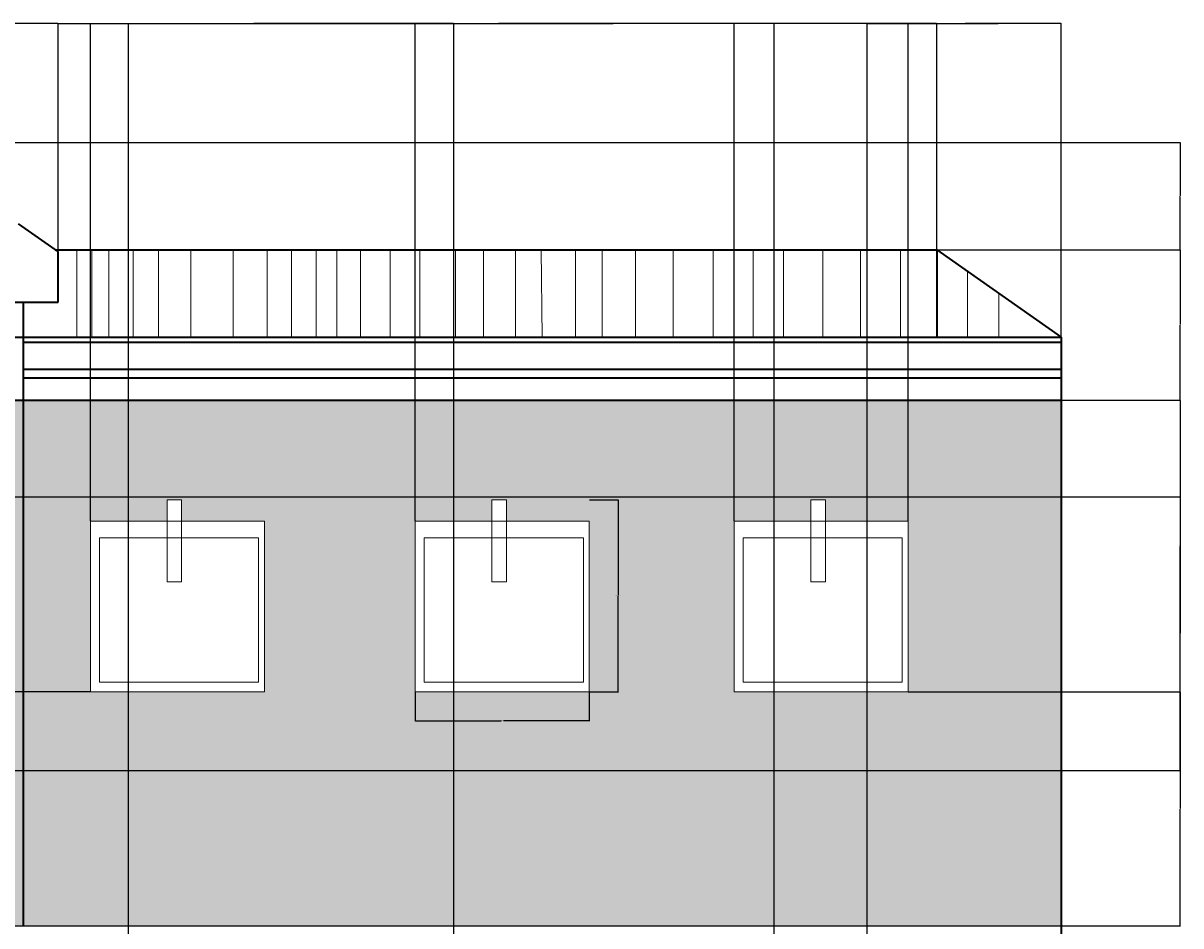
# Model space of a CAD drawing. Units: inches. Extents: x -46 to 1209, y 110 to 778.
# Tile 5 of 5: x 652 to 1209, y 342 to 778. Entities that reach past the tile are written whole.
import ezdxf

# ---------------------------------------------------------------- set-up
doc = ezdxf.new("R2010")
doc.units = ezdxf.units.IN
doc.header["$MEASUREMENT"] = 0
for name, color, linetype, lineweight in [('A-ANNO-DIMS', 2, 'Continuous', 18), ('A-GLAZ', 4, 'Continuous', 20), ('A-ROOF', 7, 'Continuous', 35), ('A-ROOF-PATT', 8, 'Continuous', 13), ('A-WALL', 7, 'Continuous', 35), ('A-WALL-PATT', 252, 'Continuous', 13), ('A-WALL-TRIM', 42, 'Continuous', 25)]:
    doc.layers.add(name, color=color, linetype=linetype, lineweight=lineweight)
doc.styles.get("Standard").update_dxf_attribs({"font": 'arial.ttf'})
doc.dimstyles.get("Standard").update_dxf_attribs({"dimtxt": 0.18, "dimasz": 0.18, "dimexe": 0.18, "dimexo": 0.0625, "dimgap": 0.09, "dimtad": 0, "dimtih": 1, "dimtoh": 1, "dimdec": 4, "dimzin": 0, "dimdsep": 46, "dimtxsty": 'Standard', "dimcen": 0.09, "dimadec": 0, "dimazin": 0, "dimtfac": 1, "dimtdec": 4, "dimtofl": 0, "dimtmove": 0, "dimatfit": 3, "dimfxl": 1, "dimtolj": 1, "dimtzin": 0, "dimarcsym": 0})

# ---------------------------------------------------------------- blocks, each defined once
blk = doc.blocks.new('WIN-PICTURE-KEYED')
for points in [[(36.92, 92.56), (43.93, 92.56), (43.93, 53.11), (36.92, 53.11)], [(0, 82.4), (83.85, 82.4), (83.85, 0), (0, 0)], [(4.35, 74.22), (81.02, 74.22), (81.02, 4.7), (4.35, 4.7)]]:
    blk.add_lwpolyline(points, close=True)
blk = doc.blocks.new('*D18')
at = {"layer": 'A-ANNO-DIMS', "color": 0, "lineweight": -2, "transparency": 16777216}
for p, q in [((924.42, 547.65), (938.42, 547.65)), ((938.24, 547.47), (938.24, 501.55)), ((938.24, 455.26), (938.24, 501.18)), ((924.42, 455.08), (938.42, 455.08))]:
    blk.add_line(p, q, dxfattribs=at)
at = {"layer": 'A-ANNO-DIMS', "color": 0, "transparency": 16777216}
for points in [[(938.21, 547.47), (938.27, 547.47), (938.24, 547.65)], [(938.21, 455.26), (938.27, 455.26), (938.24, 455.08)]]:
    blk.add_solid(points, dxfattribs=at)
at = {"layer": 'Defpoints', "color": 0, "transparency": 16777216}
for p in [(924.36, 547.65), (938.24, 547.65), (924.36, 455.08)]:
    blk.add_point(p, dxfattribs=at)
at = {"layer": 'A-ANNO-DIMS', "color": 0, "transparency": 16777216, "insert": (938.24, 501.36), "char_height": 0.18, "attachment_point": 5}
blk.add_mtext('\\A1;PICTURE WINDOW 93 TYP.', dxfattribs=at)
blk = doc.blocks.new('*D19')
at = {"layer": 'A-ANNO-DIMS', "color": 0, "lineweight": -2, "transparency": 16777216}
for p, q in [((840.5, 455.02), (840.5, 441.02)), ((924.36, 455.02), (924.36, 441.02)), ((840.68, 441.2), (881.9, 441.2)), ((924.18, 441.2), (882.96, 441.2))]:
    blk.add_line(p, q, dxfattribs=at)
at = {"layer": 'A-ANNO-DIMS', "color": 0, "transparency": 16777216}
for points in [[(840.68, 441.23), (840.68, 441.17), (840.5, 441.2)], [(924.18, 441.23), (924.18, 441.17), (924.36, 441.2)]]:
    blk.add_solid(points, dxfattribs=at)
at = {"layer": 'Defpoints', "color": 0, "transparency": 16777216}
for p in [(840.5, 455.08), (924.36, 455.08), (924.36, 441.2)]:
    blk.add_point(p, dxfattribs=at)
at = {"layer": 'A-ANNO-DIMS', "color": 0, "transparency": 16777216, "insert": (882.43, 441.2), "char_height": 0.18, "attachment_point": 5}
blk.add_mtext('\\A1;84 TYP.', dxfattribs=at)
blk = doc.blocks.new('*D56')
at = {"layer": 'A-ANNO-DIMS', "color": 0, "lineweight": -2, "transparency": 16777216}
for p, q in [((1078.14, 455.08), (1209.28, 455.08)), ((1209.1, 454.9), (1209.1, 398.86)), ((1209.1, 342.44), (1209.1, 398.49)), ((1151.86, 342.26), (1209.28, 342.26))]:
    blk.add_line(p, q, dxfattribs=at)
at = {"layer": 'A-ANNO-DIMS', "color": 0, "transparency": 16777216}
for points in [[(1209.07, 454.9), (1209.13, 454.9), (1209.1, 455.08)], [(1209.07, 342.44), (1209.13, 342.44), (1209.1, 342.26)]]:
    blk.add_solid(points, dxfattribs=at)
at = {"layer": 'Defpoints', "color": 0, "transparency": 16777216}
for p in [(1078.08, 455.08), (1209.1, 455.08), (1151.8, 342.26)]:
    blk.add_point(p, dxfattribs=at)
at = {"layer": 'A-ANNO-DIMS', "color": 0, "transparency": 16777216, "insert": (1209.1, 398.67), "char_height": 0.18, "attachment_point": 5}
blk.add_mtext('\\A1;112.82', dxfattribs=at)
blk = doc.blocks.new('*D57')
at = {"layer": 'A-ANNO-DIMS', "color": 0, "lineweight": -2, "transparency": 16777216}
for p, q in [((1151.86, 595.79), (1209.28, 595.79)), ((1209.1, 595.61), (1209.1, 525.62)), ((1209.1, 455.26), (1209.1, 525.26)), ((1078.14, 455.08), (1209.28, 455.08))]:
    blk.add_line(p, q, dxfattribs=at)
at = {"layer": 'A-ANNO-DIMS', "color": 0, "transparency": 16777216}
for points in [[(1209.07, 595.61), (1209.13, 595.61), (1209.1, 595.79)], [(1209.07, 455.26), (1209.13, 455.26), (1209.1, 455.08)]]:
    blk.add_solid(points, dxfattribs=at)
at = {"layer": 'Defpoints', "color": 0, "transparency": 16777216}
for p in [(1151.8, 595.79), (1209.1, 595.79), (1078.08, 455.08)]:
    blk.add_point(p, dxfattribs=at)
at = {"layer": 'A-ANNO-DIMS', "color": 0, "transparency": 16777216, "insert": (1209.1, 525.44), "char_height": 0.18, "attachment_point": 5}
blk.add_mtext('\\A1;140.7', dxfattribs=at)
blk = doc.blocks.new('*D58')
at = {"layer": 'A-ANNO-DIMS', "color": 0, "lineweight": -2, "transparency": 16777216}
for p, q in [((1091.9, 668.3), (1209.28, 668.3)), ((1209.1, 668.12), (1209.1, 632.23)), ((1209.1, 595.97), (1209.1, 631.86)), ((1151.86, 595.79), (1209.28, 595.79))]:
    blk.add_line(p, q, dxfattribs=at)
at = {"layer": 'A-ANNO-DIMS', "color": 0, "transparency": 16777216}
for points in [[(1209.07, 668.12), (1209.13, 668.12), (1209.1, 668.3)], [(1209.07, 595.97), (1209.13, 595.97), (1209.1, 595.79)]]:
    blk.add_solid(points, dxfattribs=at)
at = {"layer": 'Defpoints', "color": 0, "transparency": 16777216}
for p in [(1091.84, 668.3), (1209.1, 668.3), (1151.8, 595.79)]:
    blk.add_point(p, dxfattribs=at)
at = {"layer": 'A-ANNO-DIMS', "color": 0, "transparency": 16777216, "insert": (1209.1, 632.05), "char_height": 0.18, "attachment_point": 5}
blk.add_mtext('\\A1;72.51', dxfattribs=at)
blk = doc.blocks.new('*D59')
at = {"layer": 'A-ANNO-DIMS', "color": 0, "lineweight": -2, "transparency": 16777216}
for p, q in [((530.31, 720.07), (1209.28, 720.07)), ((1209.1, 719.89), (1209.1, 694.37)), ((1209.1, 668.48), (1209.1, 694)), ((1091.9, 668.3), (1209.28, 668.3))]:
    blk.add_line(p, q, dxfattribs=at)
at = {"layer": 'A-ANNO-DIMS', "color": 0, "transparency": 16777216}
for points in [[(1209.07, 719.89), (1209.13, 719.89), (1209.1, 720.07)], [(1209.07, 668.48), (1209.13, 668.48), (1209.1, 668.3)]]:
    blk.add_solid(points, dxfattribs=at)
at = {"layer": 'Defpoints', "color": 0, "transparency": 16777216}
for p in [(530.25, 720.07), (1209.1, 720.07), (1091.84, 668.3)]:
    blk.add_point(p, dxfattribs=at)
at = {"layer": 'A-ANNO-DIMS', "color": 0, "transparency": 16777216, "insert": (1209.1, 694.19), "char_height": 0.18, "attachment_point": 5}
blk.add_mtext('\\A1;51.77', dxfattribs=at)
blk = doc.blocks.new('*D66')
at = {"layer": 'A-ANNO-DIMS', "color": 0, "lineweight": -2, "transparency": 16777216}
for p, q in [((575.99, 549.2), (1209.28, 549.2)), ((1209.1, 549.02), (1209.1, 483.35)), ((1209.1, 417.31), (1209.1, 482.99)), ((575.99, 417.13), (1209.28, 417.13))]:
    blk.add_line(p, q, dxfattribs=at)
at = {"layer": 'A-ANNO-DIMS', "color": 0, "transparency": 16777216}
for points in [[(1209.07, 549.02), (1209.13, 549.02), (1209.1, 549.2)], [(1209.07, 417.31), (1209.13, 417.31), (1209.1, 417.13)]]:
    blk.add_solid(points, dxfattribs=at)
at = {"layer": 'Defpoints', "color": 0, "transparency": 16777216}
for p in [(575.92, 549.2), (1209.1, 549.2), (575.92, 417.13)]:
    blk.add_point(p, dxfattribs=at)
at = {"layer": 'A-ANNO-DIMS', "color": 0, "transparency": 16777216, "insert": (1209.1, 483.17), "char_height": 0.18, "attachment_point": 5}
blk.add_mtext('\\A1;132.07', dxfattribs=at)
blk = doc.blocks.new('*D67')
at = {"layer": 'A-ANNO-DIMS', "color": 0, "lineweight": -2, "transparency": 16777216}
for p, q in [((683.9, 455.08), (-45.5, 455.08)), ((-45.32, 454.9), (-45.32, 436.29)), ((-45.32, 417.31), (-45.32, 435.93)), ((575.86, 417.13), (-45.5, 417.13))]:
    blk.add_line(p, q, dxfattribs=at)
at = {"layer": 'A-ANNO-DIMS', "color": 0, "transparency": 16777216}
for points in [[(-45.35, 454.9), (-45.29, 454.9), (-45.32, 455.08)], [(-45.35, 417.31), (-45.29, 417.31), (-45.32, 417.13)]]:
    blk.add_solid(points, dxfattribs=at)
at = {"layer": 'Defpoints', "color": 0, "transparency": 16777216}
for p in [(-45.32, 455.08), (683.96, 455.08), (575.92, 417.13)]:
    blk.add_point(p, dxfattribs=at)
at = {"layer": 'A-ANNO-DIMS', "color": 0, "transparency": 16777216, "insert": (-45.32, 436.11), "char_height": 0.18, "attachment_point": 5}
blk.add_mtext('\\A1;37.95', dxfattribs=at)
blk = doc.blocks.new('*D68')
at = {"layer": 'A-ANNO-DIMS', "color": 0, "lineweight": -2, "transparency": 16777216}
for p, q in [((683.96, 537.54), (683.96, 777.55)), ((684.14, 777.37), (761.78, 777.37)), ((840.32, 777.37), (762.69, 777.37)), ((840.5, 537.54), (840.5, 777.55))]:
    blk.add_line(p, q, dxfattribs=at)
at = {"layer": 'A-ANNO-DIMS', "color": 0, "transparency": 16777216}
for points in [[(684.14, 777.4), (684.14, 777.34), (683.96, 777.37)], [(840.32, 777.4), (840.32, 777.34), (840.5, 777.37)]]:
    blk.add_solid(points, dxfattribs=at)
at = {"layer": 'Defpoints', "color": 0, "transparency": 16777216}
for p in [(840.5, 777.37), (683.96, 537.48), (840.5, 537.48)]:
    blk.add_point(p, dxfattribs=at)
at = {"layer": 'A-ANNO-DIMS', "color": 0, "transparency": 16777216, "insert": (762.23, 777.37), "char_height": 0.18, "attachment_point": 5}
blk.add_mtext('\\A1;156.54', dxfattribs=at)
blk = doc.blocks.new('*D69')
at = {"layer": 'A-ANNO-DIMS', "color": 0, "lineweight": -2, "transparency": 16777216}
for p, q in [((840.5, 537.54), (840.5, 777.55)), ((840.68, 777.37), (916.91, 777.37)), ((994.04, 777.37), (917.82, 777.37)), ((994.22, 537.54), (994.22, 777.55))]:
    blk.add_line(p, q, dxfattribs=at)
at = {"layer": 'A-ANNO-DIMS', "color": 0, "transparency": 16777216}
for points in [[(840.68, 777.4), (840.68, 777.34), (840.5, 777.37)], [(994.04, 777.4), (994.04, 777.34), (994.22, 777.37)]]:
    blk.add_solid(points, dxfattribs=at)
at = {"layer": 'Defpoints', "color": 0, "transparency": 16777216}
for p in [(994.22, 777.37), (840.5, 537.48), (994.22, 537.48)]:
    blk.add_point(p, dxfattribs=at)
at = {"layer": 'A-ANNO-DIMS', "color": 0, "transparency": 16777216, "insert": (917.36, 777.37), "char_height": 0.18, "attachment_point": 5}
blk.add_mtext('\\A1;153.72', dxfattribs=at)
blk = doc.blocks.new('*D70')
at = {"layer": 'A-ANNO-DIMS', "color": 0, "lineweight": -2, "transparency": 16777216}
for p, q in [((1078.08, 537.54), (1078.08, 777.55)), ((1078.26, 777.37), (1114.55, 777.37)), ((1151.62, 777.37), (1115.33, 777.37)), ((1151.8, 595.85), (1151.8, 777.55))]:
    blk.add_line(p, q, dxfattribs=at)
at = {"layer": 'A-ANNO-DIMS', "color": 0, "transparency": 16777216}
for points in [[(1078.26, 777.4), (1078.26, 777.34), (1078.08, 777.37)], [(1151.62, 777.4), (1151.62, 777.34), (1151.8, 777.37)]]:
    blk.add_solid(points, dxfattribs=at)
at = {"layer": 'Defpoints', "color": 0, "transparency": 16777216}
for p in [(1151.8, 777.37), (1151.8, 595.79), (1078.08, 537.48)]:
    blk.add_point(p, dxfattribs=at)
at = {"layer": 'A-ANNO-DIMS', "color": 0, "transparency": 16777216, "insert": (1114.94, 777.37), "char_height": 0.18, "attachment_point": 5}
blk.add_mtext('\\A1;73.72', dxfattribs=at)
blk = doc.blocks.new('*D71')
at = {"layer": 'A-ANNO-DIMS', "color": 0, "lineweight": -2, "transparency": 16777216}
for p, q in [((702.3, 292.96), (702.3, 777.55)), ((702.48, 777.37), (780.23, 777.37)), ((858.88, 777.37), (781.14, 777.37)), ((859.06, 292.96), (859.06, 777.55))]:
    blk.add_line(p, q, dxfattribs=at)
at = {"layer": 'A-ANNO-DIMS', "color": 0, "transparency": 16777216}
for points in [[(702.48, 777.4), (702.48, 777.34), (702.3, 777.37)], [(858.88, 777.4), (858.88, 777.34), (859.06, 777.37)]]:
    blk.add_solid(points, dxfattribs=at)
at = {"layer": 'Defpoints', "color": 0, "transparency": 16777216}
for p in [(859.06, 777.37), (702.3, 292.89), (859.06, 292.89)]:
    blk.add_point(p, dxfattribs=at)
at = {"layer": 'A-ANNO-DIMS', "color": 0, "transparency": 16777216, "insert": (780.68, 777.37), "char_height": 0.18, "attachment_point": 5}
blk.add_mtext('\\A1;156.76', dxfattribs=at)
blk = doc.blocks.new('*D72')
at = {"layer": 'A-ANNO-DIMS', "color": 0, "lineweight": -2, "transparency": 16777216}
for p, q in [((859.06, 292.96), (859.06, 777.55)), ((859.24, 777.37), (935.87, 777.37)), ((1013.27, 777.37), (936.64, 777.37)), ((1013.45, 292.96), (1013.45, 777.55))]:
    blk.add_line(p, q, dxfattribs=at)
at = {"layer": 'A-ANNO-DIMS', "color": 0, "transparency": 16777216}
for points in [[(859.24, 777.4), (859.24, 777.34), (859.06, 777.37)], [(1013.27, 777.4), (1013.27, 777.34), (1013.45, 777.37)]]:
    blk.add_solid(points, dxfattribs=at)
at = {"layer": 'Defpoints', "color": 0, "transparency": 16777216}
for p in [(1013.45, 777.37), (859.06, 292.89), (1013.45, 292.89)]:
    blk.add_point(p, dxfattribs=at)
at = {"layer": 'A-ANNO-DIMS', "color": 0, "transparency": 16777216, "insert": (936.26, 777.37), "char_height": 0.18, "attachment_point": 5}
blk.add_mtext('\\A1;154.4', dxfattribs=at)
blk = doc.blocks.new('*D73')
at = {"layer": 'A-ANNO-DIMS', "color": 0, "lineweight": -2, "transparency": 16777216}
for p, q in [((1058.36, 292.85), (1058.36, 777.55)), ((1058.54, 777.37), (1104.69, 777.37)), ((1151.62, 777.37), (1105.47, 777.37)), ((1151.8, 322.05), (1151.8, 777.55))]:
    blk.add_line(p, q, dxfattribs=at)
at = {"layer": 'A-ANNO-DIMS', "color": 0, "transparency": 16777216}
for points in [[(1058.54, 777.4), (1058.54, 777.34), (1058.36, 777.37)], [(1151.62, 777.4), (1151.62, 777.34), (1151.8, 777.37)]]:
    blk.add_solid(points, dxfattribs=at)
at = {"layer": 'Defpoints', "color": 0, "transparency": 16777216}
for p in [(1151.8, 777.37), (1151.8, 321.99), (1058.36, 292.79)]:
    blk.add_point(p, dxfattribs=at)
at = {"layer": 'A-ANNO-DIMS', "color": 0, "transparency": 16777216, "insert": (1105.08, 777.37), "char_height": 0.18, "attachment_point": 5}
blk.add_mtext('\\A1;93.44', dxfattribs=at)
blk = doc.blocks.new('*D78')
at = {"layer": 'A-ANNO-DIMS', "color": 0, "lineweight": -2, "transparency": 16777216}
for p, q in [((366.79, 643.05), (366.79, 777.55)), ((366.97, 777.37), (517.24, 777.37)), ((668.29, 777.37), (518.02, 777.37)), ((668.47, 643.05), (668.47, 777.55))]:
    blk.add_line(p, q, dxfattribs=at)
at = {"layer": 'A-ANNO-DIMS', "color": 0, "transparency": 16777216}
for points in [[(366.97, 777.4), (366.97, 777.34), (366.79, 777.37)], [(668.29, 777.4), (668.29, 777.34), (668.47, 777.37)]]:
    blk.add_solid(points, dxfattribs=at)
at = {"layer": 'Defpoints', "color": 0, "transparency": 16777216}
for p in [(668.47, 777.37), (366.79, 642.99), (668.47, 642.99)]:
    blk.add_point(p, dxfattribs=at)
at = {"layer": 'A-ANNO-DIMS', "color": 0, "transparency": 16777216, "insert": (517.63, 777.37), "char_height": 0.18, "attachment_point": 5}
blk.add_mtext('\\A1;301.7', dxfattribs=at)
blk = doc.blocks.new('*D79')
at = {"layer": 'A-ANNO-DIMS', "color": 0, "lineweight": -2, "transparency": 16777216}
for p, q in [((668.47, 667.37), (668.47, 777.55)), ((668.65, 777.37), (879.76, 777.37)), ((1091.66, 777.37), (880.55, 777.37)), ((1091.84, 668.36), (1091.84, 777.55))]:
    blk.add_line(p, q, dxfattribs=at)
at = {"layer": 'A-ANNO-DIMS', "color": 0, "transparency": 16777216}
for points in [[(668.65, 777.4), (668.65, 777.34), (668.47, 777.37)], [(1091.66, 777.4), (1091.66, 777.34), (1091.84, 777.37)]]:
    blk.add_solid(points, dxfattribs=at)
at = {"layer": 'Defpoints', "color": 0, "transparency": 16777216}
for p in [(1091.84, 777.37), (668.47, 667.31), (1091.84, 668.3)]:
    blk.add_point(p, dxfattribs=at)
at = {"layer": 'A-ANNO-DIMS', "color": 0, "transparency": 16777216, "insert": (880.15, 777.37), "char_height": 0.18, "attachment_point": 5}
blk.add_mtext('\\A1;423.4', dxfattribs=at)
blk = doc.blocks.new('*D80')
at = {"layer": 'A-ANNO-DIMS', "color": 0, "lineweight": -2, "transparency": 16777216}
for p, q in [((1091.84, 668.36), (1091.84, 777.55)), ((1092.02, 777.37), (1121.43, 777.37)), ((1151.62, 777.37), (1122.21, 777.37)), ((1151.8, 626.19), (1151.8, 777.55))]:
    blk.add_line(p, q, dxfattribs=at)
at = {"layer": 'A-ANNO-DIMS', "color": 0, "transparency": 16777216}
for points in [[(1092.02, 777.4), (1092.02, 777.34), (1091.84, 777.37)], [(1151.62, 777.4), (1151.62, 777.34), (1151.8, 777.37)]]:
    blk.add_solid(points, dxfattribs=at)
at = {"layer": 'Defpoints', "color": 0, "transparency": 16777216}
for p in [(1151.8, 777.37), (1091.84, 668.3), (1151.8, 626.13)]:
    blk.add_point(p, dxfattribs=at)
at = {"layer": 'A-ANNO-DIMS', "color": 0, "transparency": 16777216, "insert": (1121.82, 777.37), "char_height": 0.18, "attachment_point": 5}
blk.add_mtext('\\A1;59.96', dxfattribs=at)

msp = doc.modelspace()

# ---------------------------------------------------------------- hatches: boundary and pattern name
at = {"layer": 'A-WALL-PATT'}
h = msp.add_hatch(dxfattribs=at)
h.set_pattern_fill('AR-CONC', color=256, scale=3)
h.paths.add_polyline_path([(387.8322, 595.7911), (179.1007, 595.7911), (179.1007, 451.7911), (179.1007, 439.7911), (220.892, 454.7186), (313.6366, 436.1845), (387.8322, 376.346)])
h.paths.add_polyline_path([(276.7646, 548.5945), (292.8821, 548.5945), (292.8821, 553.0308), (295.9402, 553.0308), (295.9402, 548.5945), (313.3682, 548.5945), (313.3682, 512.6263), (276.7646, 512.6263)], flags=16)
h.paths.add_polyline_path([(278.6627, 545.0233), (312.1316, 545.0233), (312.1316, 514.6792), (278.6627, 514.6792)], flags=0)
h.paths.add_polyline_path([(326.2691, 548.5945), (341.5129, 548.5945), (341.5129, 553.0308), (344.571, 553.0308), (344.571, 548.5945), (362.8728, 548.5945), (362.8728, 512.6263), (326.2691, 512.6263)], flags=16)
h.paths.add_polyline_path([(328.1673, 545.0233), (361.6362, 545.0233), (361.6362, 514.6792), (328.1673, 514.6792)], flags=0)
h.paths.add_polyline_path([(651.5361, 595.7911), (415.401, 595.7911), (387.8322, 595.7911), (387.8322, 376.346), (409.6414, 342.2631), (651.5361, 342.2631)])
h.paths.add_polyline_path([(470.5081, 534.2042), (467.0793, 534.2042), (467.0793, 554.4029), (483.2058, 554.4029), (483.2058, 549.2024), (518.0634, 549.2024), (518.0634, 557.4852), (520.3257, 557.4852), (520.3257, 564.6435), (523.2165, 564.6435), (523.2165, 557.4852), (525.4788, 557.4852), (525.4788, 549.2024), (567.4184, 549.2024), (567.4184, 554.4029), (579.1691, 554.4029), (579.1691, 534.2042), (575.9249, 534.2042), (575.9249, 428.1662), (580.259, 428.1662), (580.259, 412.8567), (567.4184, 412.8567), (567.4184, 417.1318), (483.8186, 417.1318), (483.8186, 413.5449), (465.7589, 413.5449), (465.7589, 426.3336), (470.5081, 426.3336)], flags=16)
h.paths.add_polyline_path([(483.2375, 532.926), (568.2834, 532.926), (568.2834, 425.5857), (483.2375, 425.5857)], flags=0)
h.paths.add_polyline_path([(431.7717, 578.8147), (431.7717, 585.9699), (440.9467, 585.9699), (440.9467, 578.8147)], flags=16)
h.paths.add_polyline_path([(423.2681, 578.8147), (414.0931, 578.8147), (414.0931, 585.9699), (423.2681, 585.9699)], flags=16)
h.paths.add_polyline_path([(447.8839, 578.8147), (447.8839, 585.9699), (457.0589, 585.9699), (457.0589, 578.8147)], flags=16)
h.paths.add_polyline_path([(406.5964, 578.8147), (397.4214, 578.8147), (397.4214, 585.9699), (406.5964, 585.9699)], flags=16)
h.paths.add_polyline_path([(466.0101, 578.8147), (466.0101, 585.9699), (475.1851, 585.9699), (475.1851, 578.8147)], flags=16)
h.paths.add_polyline_path([(483.6888, 578.8147), (483.6888, 585.9699), (492.8638, 585.9699), (492.8638, 578.8147)], flags=16)
h.paths.add_polyline_path([(504.0528, 578.8147), (504.0528, 585.9699), (513.2278, 585.9699), (513.2278, 578.8147)], flags=16)
h.paths.add_polyline_path([(523.0742, 578.8147), (523.0742, 585.9699), (532.2492, 585.9699), (532.2492, 578.8147)], flags=16)
h.paths.add_polyline_path([(542.3193, 578.8147), (542.3193, 585.9699), (551.4943, 585.9699), (551.4943, 578.8147)], flags=16)
h.paths.add_polyline_path([(559.998, 578.8147), (559.998, 585.9699), (569.1729, 585.9699), (569.1729, 578.8147)], flags=16)
h.paths.add_polyline_path([(580.1382, 578.8147), (580.1382, 585.9699), (589.3132, 585.9699), (589.3132, 578.8147)], flags=16)
h.paths.add_polyline_path([(598.3313, 578.8147), (598.3313, 585.9699), (607.5063, 585.9699), (607.5063, 578.8147)], flags=16)
h.paths.add_polyline_path([(618.2477, 578.8147), (618.2477, 585.9699), (627.4227, 585.9699), (627.4227, 578.8147)], flags=16)
h.paths.add_polyline_path([(636.8215, 578.8147), (636.8215, 585.9699), (645.9965, 585.9699), (645.9965, 578.8147)], flags=16)
h.paths.add_polyline_path([(1151.8016, 595.7911), (651.5361, 595.7911), (651.5361, 342.2631), (939.9139, 342.2631), (1151.8016, 342.2631)])
h.paths.add_polyline_path([(683.9631, 455.0835), (683.9631, 537.4823), (720.8864, 537.4823), (720.8864, 547.6453), (727.8922, 547.6453), (727.8922, 537.4823), (767.8177, 537.4823), (767.8177, 455.0835)], flags=16)
h.paths.add_polyline_path([(688.3115, 459.7865), (688.3115, 529.3012), (764.9847, 529.3012), (764.9847, 459.7865)], flags=0)
h.paths.add_polyline_path([(840.5045, 455.0835), (840.5045, 537.4823), (877.4279, 537.4823), (877.4279, 547.6453), (884.4336, 547.6453), (884.4336, 537.4823), (924.3592, 537.4823), (924.3592, 455.0835)], flags=16)
h.paths.add_polyline_path([(844.853, 459.7865), (844.853, 529.3012), (921.5262, 529.3012), (921.5262, 459.7865)], flags=0)
h.paths.add_polyline_path([(994.2223, 455.0835), (994.2223, 537.4823), (1031.1457, 537.4823), (1031.1457, 547.6453), (1038.1514, 547.6453), (1038.1514, 537.4823), (1078.077, 537.4823), (1078.077, 455.0835)], flags=16)
h.paths.add_polyline_path([(998.5708, 459.7865), (998.5708, 529.3012), (1075.244, 529.3012), (1075.244, 459.7865)], flags=0)
h.paths.add_polyline_path([(1151.8016, 321.9907), (941.4829, 321.9907), (632.1261, 321.9907), (632.1261, 313.1625), (629.6322, 313.1625), (629.6322, 281.6236), (635.9059, 281.6236), (635.9059, 276.2471), (629.6322, 276.2471), (629.6322, 185.3878), (632.1261, 185.3878), (632.1261, 177.7316), (1151.8016, 177.7316)])
h.paths.add_polyline_path([(704.3294, 282.1806), (702.3037, 282.1806), (702.3037, 292.8947), (707.3294, 292.8947), (707.3294, 290.4743), (740.8704, 290.4743), (740.8704, 292.7856), (747.2108, 292.7856), (747.2108, 281.5404), (744.5274, 281.5404), (744.5274, 216.7007), (746.4513, 216.7007), (746.4513, 208.2103), (741.5274, 208.2103), (741.5274, 210.4615), (707.3294, 210.4615), (707.3294, 208.0997), (702.1613, 208.0997), (702.1613, 216.7007), (704.3294, 216.7007)], flags=16)
h.paths.add_polyline_path([(707.3294, 287.4743), (741.5274, 287.4743), (741.5274, 213.4615), (707.3294, 213.4615)], flags=0)
h.paths.add_polyline_path([(859.0635, 282.1806), (859.0635, 292.8947), (864.0892, 292.8947), (864.0892, 290.4743), (897.6301, 290.4743), (897.6301, 292.7856), (903.9705, 292.7856), (903.9705, 281.5404), (901.2871, 281.5404), (901.2871, 216.7007), (903.2111, 216.7007), (903.2111, 208.2103), (898.2871, 208.2103), (898.2871, 210.4615), (864.0892, 210.4615), (864.0892, 208.0997), (858.9211, 208.0997), (858.9211, 216.7007), (861.0892, 216.7007), (861.0892, 282.1806)], flags=16)
h.paths.add_polyline_path([(864.0892, 287.4743), (898.2871, 287.4743), (898.2871, 213.4615), (864.0892, 213.4615)], flags=0)
h.paths.add_polyline_path([(1013.4529, 282.1806), (1013.4529, 292.8947), (1018.4786, 292.8947), (1018.4786, 290.4743), (1052.0195, 290.4743), (1052.0195, 292.7856), (1058.3599, 292.7856), (1058.3599, 281.5404), (1055.6765, 281.5404), (1055.6765, 216.7007), (1057.6005, 216.7007), (1057.6005, 208.2103), (1052.6765, 208.2103), (1052.6765, 210.4615), (1018.4786, 210.4615), (1018.4786, 208.0997), (1013.3105, 208.0997), (1013.3105, 216.7007), (1015.4786, 216.7007), (1015.4786, 282.1806)], flags=16)
h.paths.add_polyline_path([(1018.4786, 287.4743), (1052.6765, 287.4743), (1052.6765, 213.4615), (1018.4786, 213.4615)], flags=0)
h.paths.add_polyline_path([(431.9367, 276.2471), (423.7231, 276.2471), (423.7231, 281.6236), (431.9367, 281.6236), (431.9367, 313.1625), (430.3199, 313.1625), (430.3199, 321.9907), (406.6462, 321.9907), (406.6462, 321.7316), (405.6256, 177.7316), (430.3199, 177.7316), (430.3199, 185.3878), (431.9367, 185.3878)])
h.paths.add_polyline_path([(406.6462, 321.7316), (406.6462, 321.9907), (363.2774, 321.9907), (58.5947, 321.7316), (57.7764, 206.2827), (87.7834, 206.0701), (87.7834, 290.4607), (89.9075, 293.33), (149.9611, 311.663), (149.9611, 316.8909), (153.3383, 316.8909), (153.3383, 311.1504), (213.2336, 293.3362), (215.3783, 290.4607), (215.3783, 205.1657), (246.588, 204.9445), (246.588, 290.0127), (248.7121, 292.882), (308.2509, 311.0579), (308.2509, 316.0122), (311.6281, 316.0122), (311.6281, 310.8556), (372.0381, 292.8882), (374.1829, 290.0127), (374.1829, 204.0402), (405.8105, 203.8161)])
h.paths.add_polyline_path([(333, 359.5), (292.5, 377), (250.5, 387.5), (199, 387.5), (155, 377.5), (123.5, 364), (101.4287, 342.2631), (363.2774, 342.2631)])
h.paths.add_polyline_path([(579.9721, 681.6773), (549.8011, 690.7996), (524.9646, 691.17), (482.8908, 691.7975), (447.0968, 679.2482), (416.3264, 659.1694), (597.1807, 659.1694)])

# ---------------------------------------------------------------- linework, layer by layer
at = {"layer": 'A-ROOF'}
for p, q in [((649.1949, 680.732), (668.4684, 667.3071)), ((667.0402, 668.3019), (1091.8408, 668.3019)), ((668.4684, 642.9876), (668.4684, 667.3071)), ((1091.8408, 668.3019), (1151.8016, 626.1254)), ((1091.8408, 668.3019), (1091.8408, 626.1254)), ((646.6805, 642.9876), (651.5361, 642.9876)), ((651.5361, 642.9876), (651.5361, 626.1254)), ((651.5361, 642.9876), (668.4684, 642.9876)), ((387.8322, 626.1254), (651.5361, 626.1254)), ((651.5361, 626.1254), (651.5361, 586.7801)), ((651.5361, 626.1254), (1151.8016, 626.1254)), ((1151.8016, 626.1254), (1151.8016, 610.7581)), ((651.5361, 623.7049), (1151.8016, 623.7049)), ((651.5361, 610.7581), (1151.8016, 610.7581)), ((1151.8016, 610.7581), (1151.8016, 606.4528)), ((651.5361, 606.4528), (1151.8016, 606.4528)), ((1151.8016, 606.4528), (1151.8016, 595.7911))]:
    msp.add_line(p, q, dxfattribs=at)
at = {"layer": 'A-ROOF-PATT'}
for p, q in [((677.4239, 668.3019), (677.4239, 626.1254)), ((684.5632, 668.3019), (684.5632, 626.1254)), ((692.7733, 668.3019), (692.7733, 626.1254)), ((704.5531, 668.3019), (704.5531, 626.1254)), ((716.6899, 668.3019), (716.6899, 626.1254)), ((732.3963, 668.3019), (732.3963, 626.1254)), ((752.7432, 668.3019), (752.7432, 626.1254)), ((769.1636, 668.3019), (769.1636, 626.1254)), ((780.9434, 668.3019), (780.9434, 626.1254)), ((792.7232, 668.3019), (792.7232, 626.1254)), ((802.7181, 668.3019), (802.7181, 626.1254)), ((814.141, 668.3019), (814.141, 626.1254)), ((828.4195, 668.3019), (828.4195, 626.1254)), ((842.6981, 668.3019), (842.6981, 626.1254)), ((859.8323, 668.3019), (859.8323, 626.1254)), ((873.397, 668.3019), (873.397, 626.1254)), ((888.7464, 668.3019), (888.7464, 626.1254)), ((901.2401, 668.3019), (901.6689, 626.1254)), ((917.6605, 668.3019), (917.6605, 626.1254)), ((930.5591, 668.3019), (930.5591, 626.1254)), ((946.6225, 668.3019), (946.6225, 626.1254)), ((964.8276, 668.3019), (964.8276, 626.1254)), ((984.1036, 668.3019), (984.1036, 626.1254)), ((1003.3797, 668.3019), (1003.3797, 626.1254)), ((1018.0152, 668.3019), (1018.0152, 626.1254)), ((1036.9342, 668.3019), (1036.9342, 626.1254)), ((1055.1394, 668.3019), (1055.1394, 626.1254)), ((1074.4154, 668.3019), (1074.4154, 626.1254)), ((1106.6356, 657.8952), (1106.6356, 626.1254)), ((1121.8212, 647.2137), (1121.8212, 626.1254))]:
    msp.add_line(p, q, dxfattribs=at)
at = {"layer": 'A-WALL'}
for p, q in [((415.401, 595.7911), (651.5361, 595.7911)), ((651.5361, 595.7911), (651.5361, 342.2631)), ((651.5361, 595.7911), (1151.8016, 595.7911)), ((1151.8016, 595.7911), (1151.8016, 177.7316))]:
    msp.add_line(p, q, dxfattribs=at)
at = {"layer": 'A-WALL-TRIM'}
for p, q in [((409.6414, 342.2631), (939.9139, 342.2631)), ((939.9139, 342.2631), (1151.8016, 342.2631))]:
    msp.add_line(p, q, dxfattribs=at)

# ---------------------------------------------------------------- block references
at = {"layer": 'A-GLAZ'}
for p in [(683.9631, 455.0835), (840.5045, 455.0835), (994.2223, 455.0835)]:
    msp.add_blockref('WIN-PICTURE-KEYED', p, dxfattribs=at)

# ---------------------------------------------------------------- dimensions: what is measured, and where the dimension line sits
at = {"layer": 'A-ANNO-DIMS'}
for base, p1, p2, override, picture, middle in [((668.4684, 777.3699), (366.7938, 642.9876), (668.4684, 642.9876), {"dimdec": 1, "dimlfac": 1, "dimrnd": 0, "dimzin": 0, "dimdsep": 46, "dimlunit": 2}, '*D78', (517.6311, 777.3699)), ((1091.8408, 777.3699), (668.4684, 667.3071), (1091.8408, 668.3019), {"dimdec": 1, "dimlfac": 1, "dimrnd": 0, "dimzin": 0, "dimdsep": 46, "dimlunit": 2}, '*D79', (880.1546, 777.3699)), ((840.5045, 777.3699), (683.9631, 537.4823), (840.5045, 537.4823), {"dimdec": 2, "dimlfac": 1, "dimrnd": 0, "dimzin": 0, "dimdsep": 46, "dimlunit": 2}, '*D68', (762.2338, 777.3699)), ((859.0635, 777.3699), (702.3037, 292.8947), (859.0635, 292.8947), {"dimdec": 2, "dimlfac": 1, "dimrnd": 0, "dimzin": 0, "dimdsep": 46, "dimlunit": 2}, '*D71', (780.6836, 777.3699)), ((994.2223, 777.3699), (840.5045, 537.4823), (994.2223, 537.4823), {"dimdec": 2, "dimlfac": 1, "dimrnd": 0, "dimzin": 0, "dimdsep": 46, "dimlunit": 2}, '*D69', (917.3634, 777.3699)), ((1013.4529, 777.3699), (859.0635, 292.8947), (1013.4529, 292.8947), {"dimdec": 1, "dimlfac": 1, "dimrnd": 0, "dimzin": 0, "dimdsep": 46, "dimlunit": 2}, '*D72', (936.2582, 777.3699)), ((1151.8016, 777.3699), (1058.3599, 292.7856), (1151.8016, 321.9907), {"dimdec": 2, "dimlfac": 1, "dimrnd": 0, "dimzin": 0, "dimdsep": 46, "dimlunit": 2}, '*D73', (1105.0807, 777.3699)), ((1151.8016, 777.3699), (1078.077, 537.4823), (1151.8016, 595.7911), {"dimdec": 2, "dimlfac": 1, "dimrnd": 0, "dimzin": 0, "dimdsep": 46, "dimlunit": 2}, '*D70', (1114.9393, 777.3699)), ((1151.8016, 777.3699), (1091.8408, 668.3019), (1151.8016, 626.1254), {"dimdec": 2, "dimlfac": 1, "dimrnd": 0, "dimzin": 0, "dimdsep": 46, "dimlunit": 2}, '*D80', (1121.8212, 777.3699))]:
    dim = msp.add_linear_dim(base=base, p1=p1, p2=p2, dimstyle='Standard', override=override, dxfattribs=at)
    dim.commit()
    dim.dimension.update_dxf_attribs({"geometry": picture, "text_midpoint": middle})
for base, p1, p2, override, picture, middle in [((1209.1016, 720.0699), (1091.8408, 668.3019), (530.2452, 720.0699), {"dimdec": 2, "dimlfac": 1, "dimrnd": 0, "dimzin": 0, "dimdsep": 46, "dimlunit": 2}, '*D59', (1209.1016, 694.1859)), ((1209.1016, 668.3019), (1151.8016, 595.7911), (1091.8408, 668.3019), {"dimdec": 2, "dimlfac": 1, "dimrnd": 0, "dimzin": 0, "dimdsep": 46, "dimlunit": 2}, '*D58', (1209.1016, 632.0465)), ((1209.1016, 595.7911), (1078.077, 455.0835), (1151.8016, 595.7911), {"dimdec": 1, "dimlfac": 1, "dimrnd": 0, "dimzin": 0, "dimdsep": 46, "dimlunit": 2}, '*D57', (1209.1016, 525.4373)), ((1209.1016, 549.2024), (575.9249, 417.1318), (575.9249, 549.2024), {"dimdec": 2, "dimlfac": 1, "dimrnd": 0, "dimzin": 0, "dimdsep": 46, "dimlunit": 2}, '*D66', (1209.1016, 483.1671)), ((-45.3158, 455.0835), (575.9249, 417.1318), (683.9631, 455.0835), {"dimdec": 2, "dimlfac": 1, "dimrnd": 0, "dimzin": 0, "dimdsep": 46, "dimlunit": 2}, '*D67', (-45.3158, 436.1076)), ((1209.1016, 455.0835), (1151.8016, 342.2631), (1078.077, 455.0835), {"dimdec": 2, "dimlfac": 1, "dimrnd": 0, "dimzin": 0, "dimdsep": 46, "dimlunit": 2}, '*D56', (1209.1016, 398.6733))]:
    dim = msp.add_linear_dim(base=base, p1=p1, p2=p2, angle=90, dimstyle='Standard', override=override, dxfattribs=at)
    dim.commit()
    dim.dimension.update_dxf_attribs({"geometry": picture, "text_midpoint": middle})
dim = msp.add_linear_dim(base=(938.2434, 547.6453), p1=(924.3592, 455.0835), p2=(924.3592, 547.6453), angle=90, text='PICTURE WINDOW <> TYP.', dimstyle='Standard', override={"dimdec": 0, "dimlfac": 1, "dimrnd": 0, "dimzin": 0, "dimdsep": 46, "dimlunit": 2}, dxfattribs=at)
dim.commit()
dim.dimension.update_dxf_attribs({"geometry": '*D18', "text_midpoint": (938.2434, 501.3644)})
dim = msp.add_linear_dim(base=(924.3592, 441.1993), p1=(840.5045, 455.0835), p2=(924.3592, 455.0835), text='<> TYP.', dimstyle='Standard', override={"dimdec": 0, "dimlfac": 1, "dimrnd": 0, "dimzin": 0, "dimdsep": 46, "dimlunit": 2}, dxfattribs=at)
dim.commit()
dim.dimension.update_dxf_attribs({"geometry": '*D19', "text_midpoint": (882.4319, 441.1993)})

doc.saveas('drawing.dxf')
